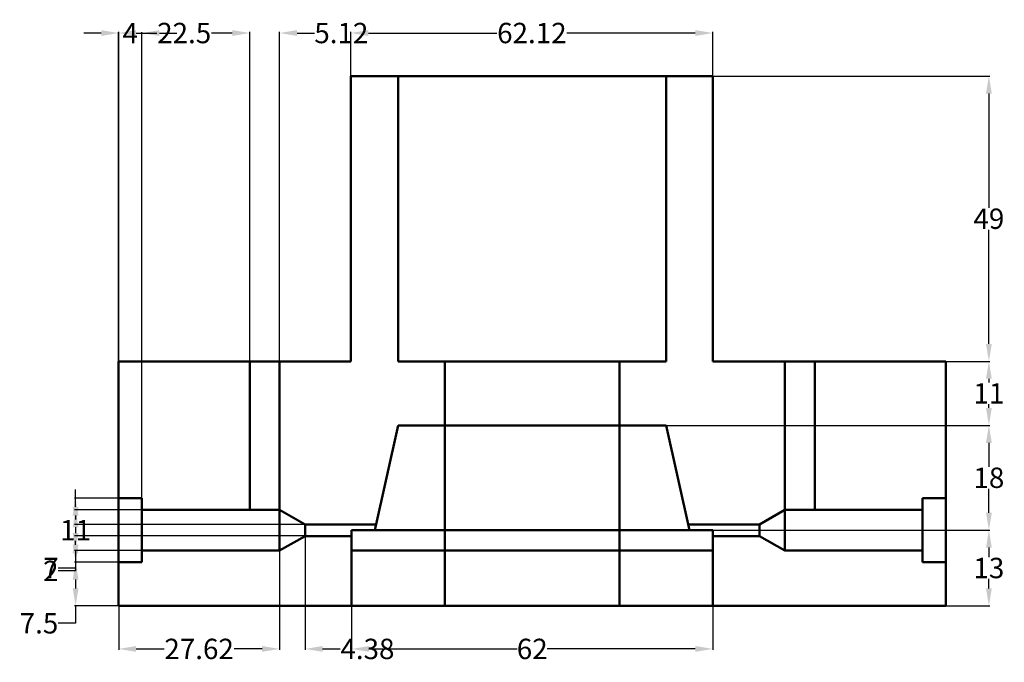
# Model space of a CAD drawing. Units: millimetres. Extents: x 646 to 860, y 238 to 552.
# Tile 1 of 2: x 646 to 815, y 238 to 349. Entities that reach past the tile are written whole.
import ezdxf

# ---------------------------------------------------------------- set-up
doc = ezdxf.new("R2010")
doc.units = ezdxf.units.MM
doc.header["$MEASUREMENT"] = 0
doc.layers.add('M-DIMS', color=2, linetype='Continuous', lineweight=18)
doc.layers.add('M-OUTL', color=7, linetype='Continuous', lineweight=50)
doc.styles.get("Standard").update_dxf_attribs({"font": 'arial.ttf'})
doc.dimstyles.get("Standard").update_dxf_attribs({"dimtxt": 3.5, "dimasz": 3, "dimexe": 0.18, "dimexo": 0.0625, "dimgap": 0.09, "dimtad": 0, "dimtih": 1, "dimtoh": 1, "dimdec": 1, "dimzin": 0, "dimdsep": 46, "dimtxsty": 'Standard', "dimcen": 0.09, "dimadec": 0, "dimazin": 0, "dimtfac": 1, "dimtdec": 1, "dimtofl": 0, "dimtmove": 0, "dimatfit": 3, "dimfxl": 1, "dimtolj": 1, "dimtzin": 0, "dimarcsym": 0})

# ---------------------------------------------------------------- blocks, each defined once
blk = doc.blocks.new('*D25')
at = {"layer": 'Defpoints', "color": 0, "transparency": 16777216}
for p in [(765.02, 261.19), (812.42, 261.19), (805.02, 248.19)]:
    blk.add_point(p, dxfattribs=at)
at = {"layer": 'M-DIMS', "color": 0, "lineweight": -2, "transparency": 16777216}
for p, q in [((765.08, 261.19), (812.6, 261.19)), ((812.42, 258.19), (812.42, 256.56)), ((812.42, 251.19), (812.42, 252.81)), ((805.08, 248.19), (812.6, 248.19))]:
    blk.add_line(p, q, dxfattribs=at)
at = {"layer": 'M-DIMS', "color": 0, "transparency": 16777216}
for points in [[(811.92, 258.19), (812.92, 258.19), (812.42, 261.19)], [(811.92, 251.19), (812.92, 251.19), (812.42, 248.19)]]:
    blk.add_solid(points, dxfattribs=at)
at = {"layer": 'M-DIMS', "color": 0, "transparency": 16777216, "insert": (812.42, 254.69), "char_height": 3.5, "attachment_point": 5}
blk.add_mtext('\\A1;13', dxfattribs=at)
blk = doc.blocks.new('*D26')
at = {"layer": 'Defpoints', "color": 0, "transparency": 16777216}
for p in [(757.02, 279.19), (812.42, 279.19), (765.02, 261.19)]:
    blk.add_point(p, dxfattribs=at)
at = {"layer": 'M-DIMS', "color": 0, "lineweight": -2, "transparency": 16777216}
for p, q in [((757.08, 279.19), (812.6, 279.19)), ((812.42, 276.19), (812.42, 272.06)), ((812.42, 264.19), (812.42, 268.31)), ((765.08, 261.19), (812.6, 261.19))]:
    blk.add_line(p, q, dxfattribs=at)
at = {"layer": 'M-DIMS', "color": 0, "transparency": 16777216}
for points in [[(811.92, 276.19), (812.92, 276.19), (812.42, 279.19)], [(811.92, 264.19), (812.92, 264.19), (812.42, 261.19)]]:
    blk.add_solid(points, dxfattribs=at)
at = {"layer": 'M-DIMS', "color": 0, "transparency": 16777216, "insert": (812.42, 270.19), "char_height": 3.5, "attachment_point": 5}
blk.add_mtext('\\A1;18', dxfattribs=at)
blk = doc.blocks.new('*D27')
at = {"layer": 'Defpoints', "color": 0, "transparency": 16777216}
for p in [(805.02, 290.19), (812.42, 290.19), (757.02, 279.19)]:
    blk.add_point(p, dxfattribs=at)
at = {"layer": 'M-DIMS', "color": 0, "lineweight": -2, "transparency": 16777216}
for p, q in [((805.08, 290.19), (812.6, 290.19)), ((812.42, 287.19), (812.42, 286.53)), ((812.42, 282.19), (812.42, 282.84)), ((757.08, 279.19), (812.6, 279.19))]:
    blk.add_line(p, q, dxfattribs=at)
at = {"layer": 'M-DIMS', "color": 0, "transparency": 16777216}
for points in [[(811.92, 287.19), (812.92, 287.19), (812.42, 290.19)], [(811.92, 282.19), (812.92, 282.19), (812.42, 279.19)]]:
    blk.add_solid(points, dxfattribs=at)
at = {"layer": 'M-DIMS', "color": 0, "transparency": 16777216, "insert": (812.42, 284.69), "char_height": 3.5, "attachment_point": 5}
blk.add_mtext('\\A1;11', dxfattribs=at)
blk = doc.blocks.new('*D28')
at = {"layer": 'Defpoints', "color": 0, "transparency": 16777216}
for p in [(765.02, 339.19), (812.42, 339.19), (805.02, 290.19)]:
    blk.add_point(p, dxfattribs=at)
at = {"layer": 'M-DIMS', "color": 0, "lineweight": -2, "transparency": 16777216}
for p, q in [((765.08, 339.19), (812.6, 339.19)), ((812.42, 336.19), (812.42, 316.56)), ((812.42, 293.19), (812.42, 312.81)), ((805.08, 290.19), (812.6, 290.19))]:
    blk.add_line(p, q, dxfattribs=at)
at = {"layer": 'M-DIMS', "color": 0, "transparency": 16777216}
for points in [[(811.92, 336.19), (812.92, 336.19), (812.42, 339.19)], [(811.92, 293.19), (812.92, 293.19), (812.42, 290.19)]]:
    blk.add_solid(points, dxfattribs=at)
at = {"layer": 'M-DIMS', "color": 0, "transparency": 16777216, "insert": (812.42, 314.69), "char_height": 3.5, "attachment_point": 5}
blk.add_mtext('\\A1;49', dxfattribs=at)
blk = doc.blocks.new('*D29')
at = {"layer": 'Defpoints', "color": 0, "transparency": 16777216}
for p in [(765.02, 346.59), (702.9, 339.19), (765.02, 339.19)]:
    blk.add_point(p, dxfattribs=at)
at = {"layer": 'M-DIMS', "color": 0, "lineweight": -2, "transparency": 16777216}
for p, q in [((702.9, 339.25), (702.9, 346.77)), ((705.9, 346.59), (727.97, 346.59)), ((762.02, 346.59), (739.94, 346.59)), ((765.02, 339.25), (765.02, 346.77))]:
    blk.add_line(p, q, dxfattribs=at)
at = {"layer": 'M-DIMS', "color": 0, "transparency": 16777216}
for points in [[(705.9, 347.09), (705.9, 346.09), (702.9, 346.59)], [(762.02, 347.09), (762.02, 346.09), (765.02, 346.59)]]:
    blk.add_solid(points, dxfattribs=at)
at = {"layer": 'M-DIMS', "color": 0, "transparency": 16777216, "insert": (733.96, 346.59), "char_height": 3.5, "attachment_point": 5}
blk.add_mtext('\\A1;62.12', dxfattribs=at)
blk = doc.blocks.new('*D30')
at = {"layer": 'Defpoints', "color": 0, "transparency": 16777216}
for p in [(703.02, 248.19), (765.02, 248.19), (765.02, 240.79)]:
    blk.add_point(p, dxfattribs=at)
at = {"layer": 'M-DIMS', "color": 0, "lineweight": -2, "transparency": 16777216}
for p, q in [((703.02, 248.12), (703.02, 240.61)), ((765.02, 248.12), (765.02, 240.61)), ((706.02, 240.79), (731.43, 240.79)), ((762.02, 240.79), (736.6, 240.79))]:
    blk.add_line(p, q, dxfattribs=at)
at = {"layer": 'M-DIMS', "color": 0, "transparency": 16777216}
for points in [[(706.02, 241.29), (706.02, 240.29), (703.02, 240.79)], [(762.02, 241.29), (762.02, 240.29), (765.02, 240.79)]]:
    blk.add_solid(points, dxfattribs=at)
at = {"layer": 'M-DIMS', "color": 0, "transparency": 16777216, "insert": (734.02, 240.79), "char_height": 3.5, "attachment_point": 5}
blk.add_mtext('\\A1;62', dxfattribs=at)
blk = doc.blocks.new('*D31')
at = {"layer": 'Defpoints', "color": 0, "transparency": 16777216}
for p in [(663.02, 266.69), (655.62, 255.69), (663.02, 255.69)]:
    blk.add_point(p, dxfattribs=at)
at = {"layer": 'M-DIMS', "color": 0, "lineweight": -2, "transparency": 16777216}
for p, q in [((662.95, 266.69), (655.44, 266.69)), ((655.62, 263.69), (655.62, 263.03)), ((655.62, 258.69), (655.62, 259.34)), ((662.95, 255.69), (655.44, 255.69))]:
    blk.add_line(p, q, dxfattribs=at)
at = {"layer": 'M-DIMS', "color": 0, "transparency": 16777216}
for points in [[(655.12, 263.69), (656.12, 263.69), (655.62, 266.69)], [(655.12, 258.69), (656.12, 258.69), (655.62, 255.69)]]:
    blk.add_solid(points, dxfattribs=at)
at = {"layer": 'M-DIMS', "color": 0, "transparency": 16777216, "insert": (655.62, 261.19), "char_height": 3.5, "attachment_point": 5}
blk.add_mtext('\\A1;11', dxfattribs=at)
blk = doc.blocks.new('*D32')
at = {"layer": 'Defpoints', "color": 0, "transparency": 16777216}
for p in [(667.015746, 346.585612), (663.015746, 266.685612), (667.015746, 266.685612)]:
    blk.add_point(p, dxfattribs=at)
at = {"layer": 'M-DIMS', "color": 0, "lineweight": -2, "transparency": 16777216}
for p, q in [((660.015746, 346.585612), (657.015746, 346.585612)), ((663.015746, 266.748112), (663.015746, 346.765612)), ((667.015746, 266.748112), (667.015746, 346.765612)), ((670.015746, 346.585612), (673.015746, 346.585612))]:
    blk.add_line(p, q, dxfattribs=at)
at = {"layer": 'M-DIMS', "color": 0, "transparency": 16777216}
for points in [[(660.015746, 347.085612), (660.015746, 346.085612), (663.015746, 346.585612)], [(670.015746, 347.085612), (670.015746, 346.085612), (667.015746, 346.585612)]]:
    blk.add_solid(points, dxfattribs=at)
at = {"layer": 'M-DIMS', "color": 0, "transparency": 16777216, "insert": (665.015746, 346.585612), "char_height": 3.5, "attachment_point": 5}
blk.add_mtext('\\A1;4', dxfattribs=at)
blk = doc.blocks.new('*D33')
at = {"layer": 'Defpoints', "color": 0, "transparency": 16777216}
for p in [(667.02, 264.69), (655.62, 257.69), (667.02, 257.69)]:
    blk.add_point(p, dxfattribs=at)
at = {"layer": 'M-DIMS', "color": 0, "lineweight": -2, "transparency": 16777216}
for p, q in [((666.95, 264.69), (655.44, 264.69)), ((655.62, 261.69), (655.62, 260.69)), ((666.95, 257.69), (655.44, 257.69)), ((655.62, 257.69), (655.62, 254.69)), ((655.62, 254.69), (652.62, 254.69))]:
    blk.add_line(p, q, dxfattribs=at)
at = {"layer": 'M-DIMS', "color": 0, "transparency": 16777216}
for points in [[(655.12, 261.69), (656.12, 261.69), (655.62, 264.69)], [(655.12, 260.69), (656.12, 260.69), (655.62, 257.69)]]:
    blk.add_solid(points, dxfattribs=at)
at = {"layer": 'M-DIMS', "color": 0, "transparency": 16777216, "insert": (651.39, 254.69), "char_height": 3.5, "attachment_point": 5}
blk.add_mtext('\\A1;7', dxfattribs=at)
blk = doc.blocks.new('*D34')
at = {"layer": 'Defpoints', "color": 0, "transparency": 16777216}
for p in [(690.64, 257.69), (663.02, 255.69), (690.64, 240.79)]:
    blk.add_point(p, dxfattribs=at)
at = {"layer": 'M-DIMS', "color": 0, "lineweight": -2, "transparency": 16777216}
for p, q in [((690.64, 257.62), (690.64, 240.61)), ((663.02, 255.62), (663.02, 240.61)), ((666.02, 240.79), (670.82, 240.79)), ((687.64, 240.79), (682.83, 240.79))]:
    blk.add_line(p, q, dxfattribs=at)
at = {"layer": 'M-DIMS', "color": 0, "transparency": 16777216}
for points in [[(666.02, 241.29), (666.02, 240.29), (663.02, 240.79)], [(687.64, 241.29), (687.64, 240.29), (690.64, 240.79)]]:
    blk.add_solid(points, dxfattribs=at)
at = {"layer": 'M-DIMS', "color": 0, "transparency": 16777216, "insert": (676.83, 240.79), "char_height": 3.5, "attachment_point": 5}
blk.add_mtext('\\A1;27.62', dxfattribs=at)
blk = doc.blocks.new('*D35')
at = {"layer": 'Defpoints', "color": 0, "transparency": 16777216}
for p in [(690.64, 264.69), (695.02, 262.19), (695.02, 240.79)]:
    blk.add_point(p, dxfattribs=at)
at = {"layer": 'M-DIMS', "color": 0, "lineweight": -2, "transparency": 16777216}
for p, q in [((690.64, 264.62), (690.64, 240.61)), ((695.02, 262.12), (695.02, 240.61)), ((687.64, 240.79), (684.64, 240.79)), ((698.02, 240.79), (701.02, 240.79))]:
    blk.add_line(p, q, dxfattribs=at)
at = {"layer": 'M-DIMS', "color": 0, "transparency": 16777216}
for points in [[(687.64, 241.29), (687.64, 240.29), (690.64, 240.79)], [(698.02, 241.29), (698.02, 240.29), (695.02, 240.79)]]:
    blk.add_solid(points, dxfattribs=at)
at = {"layer": 'M-DIMS', "color": 0, "transparency": 16777216, "insert": (705.73, 240.79), "char_height": 3.5, "attachment_point": 5}
blk.add_mtext('\\A1;4.38', dxfattribs=at)
blk = doc.blocks.new('*D36')
at = {"layer": 'Defpoints', "color": 0, "transparency": 16777216}
for p in [(695.02, 262.19), (655.62, 260.19), (695.02, 260.19)]:
    blk.add_point(p, dxfattribs=at)
at = {"layer": 'M-DIMS', "color": 0, "lineweight": -2, "transparency": 16777216}
for p, q in [((655.62, 265.19), (655.62, 268.19)), ((694.95, 262.19), (655.44, 262.19)), ((694.95, 260.19), (655.44, 260.19)), ((655.62, 257.19), (655.62, 254.19)), ((655.62, 254.19), (652.62, 254.19))]:
    blk.add_line(p, q, dxfattribs=at)
at = {"layer": 'M-DIMS', "color": 0, "transparency": 16777216}
for points in [[(655.12, 265.19), (656.12, 265.19), (655.62, 262.19)], [(655.12, 257.19), (656.12, 257.19), (655.62, 260.19)]]:
    blk.add_solid(points, dxfattribs=at)
at = {"layer": 'M-DIMS', "color": 0, "transparency": 16777216, "insert": (651.37, 254.19), "char_height": 3.5, "attachment_point": 5}
blk.add_mtext('\\A1;2', dxfattribs=at)
blk = doc.blocks.new('*D37')
at = {"layer": 'Defpoints', "color": 0, "transparency": 16777216}
for p in [(663.02, 255.69), (655.62, 248.19), (663.02, 248.19)]:
    blk.add_point(p, dxfattribs=at)
at = {"layer": 'M-DIMS', "color": 0, "lineweight": -2, "transparency": 16777216}
for p, q in [((662.95, 255.69), (655.44, 255.69)), ((655.62, 252.69), (655.62, 251.19)), ((662.95, 248.19), (655.44, 248.19)), ((655.62, 248.19), (655.62, 245.19)), ((655.62, 245.19), (652.62, 245.19))]:
    blk.add_line(p, q, dxfattribs=at)
at = {"layer": 'M-DIMS', "color": 0, "transparency": 16777216}
for points in [[(655.12, 252.69), (656.12, 252.69), (655.62, 255.69)], [(655.12, 251.19), (656.12, 251.19), (655.62, 248.19)]]:
    blk.add_solid(points, dxfattribs=at)
at = {"layer": 'M-DIMS', "color": 0, "transparency": 16777216, "insert": (649.34, 245.19), "char_height": 3.5, "attachment_point": 5}
blk.add_mtext('\\A1;7.5', dxfattribs=at)
blk = doc.blocks.new('*D38')
at = {"layer": 'Defpoints', "color": 0, "transparency": 16777216}
for p in [(690.64, 346.59), (685.52, 290.19), (690.64, 290.19)]:
    blk.add_point(p, dxfattribs=at)
at = {"layer": 'M-DIMS', "color": 0, "lineweight": -2, "transparency": 16777216}
for p, q in [((682.52, 346.59), (679.52, 346.59)), ((685.52, 290.25), (685.52, 346.77)), ((690.64, 290.25), (690.64, 346.77)), ((693.64, 346.59), (696.64, 346.59))]:
    blk.add_line(p, q, dxfattribs=at)
at = {"layer": 'M-DIMS', "color": 0, "transparency": 16777216}
for points in [[(682.52, 347.09), (682.52, 346.09), (685.52, 346.59)], [(693.64, 347.09), (693.64, 346.09), (690.64, 346.59)]]:
    blk.add_solid(points, dxfattribs=at)
at = {"layer": 'M-DIMS', "color": 0, "transparency": 16777216, "insert": (701.25, 346.59), "char_height": 3.5, "attachment_point": 5}
blk.add_mtext('\\A1;5.12', dxfattribs=at)
blk = doc.blocks.new('*D39')
at = {"layer": 'Defpoints', "color": 0, "transparency": 16777216}
for p in [(685.52, 346.59), (663.02, 290.19), (685.52, 290.19)]:
    blk.add_point(p, dxfattribs=at)
at = {"layer": 'M-DIMS', "color": 0, "lineweight": -2, "transparency": 16777216}
for p, q in [((663.02, 290.25), (663.02, 346.77)), ((666.02, 346.59), (669.59, 346.59)), ((682.52, 346.59), (678.94, 346.59)), ((685.52, 290.25), (685.52, 346.77))]:
    blk.add_line(p, q, dxfattribs=at)
at = {"layer": 'M-DIMS', "color": 0, "transparency": 16777216}
for points in [[(666.02, 347.09), (666.02, 346.09), (663.02, 346.59)], [(682.52, 347.09), (682.52, 346.09), (685.52, 346.59)]]:
    blk.add_solid(points, dxfattribs=at)
at = {"layer": 'M-DIMS', "color": 0, "transparency": 16777216, "insert": (674.27, 346.59), "char_height": 3.5, "attachment_point": 5}
blk.add_mtext('\\A1;22.5', dxfattribs=at)

msp = doc.modelspace()

# ---------------------------------------------------------------- linework, layer by layer
at = {"layer": 'M-OUTL'}
for p, q in [((765.016, 339.186), (702.896, 339.186)), ((702.896, 290.186), (702.896, 339.186)), ((711.016, 290.186), (711.016, 339.186)), ((757.016, 290.186), (757.016, 339.186)), ((765.016, 290.186), (765.016, 339.186)), ((663.016, 290.186), (663.016, 248.186)), ((690.636, 290.186), (663.016, 290.186)), ((685.516, 290.186), (685.516, 264.686)), ((702.896, 290.186), (690.636, 290.186)), ((690.636, 290.186), (690.636, 257.686)), ((757.016, 290.186), (711.016, 290.186)), ((719.016, 290.186), (719.016, 248.186)), ((749.016, 290.186), (749.016, 248.186)), ((805.016, 290.186), (765.016, 290.186)), ((777.396, 290.186), (777.396, 257.686)), ((782.516, 290.186), (782.516, 264.686)), ((805.016, 290.186), (805.016, 248.186)), ((711.016, 279.186), (707.016, 261.186)), ((757.016, 279.186), (711.016, 279.186)), ((749.016, 279.186), (757.016, 279.186)), ((757.016, 279.186), (761.016, 261.186)), ((663.016, 266.686), (667.016, 266.686)), ((667.016, 266.686), (667.016, 255.686)), ((801.016, 266.686), (801.016, 255.686)), ((805.016, 266.686), (801.016, 266.686)), ((667.016, 264.686), (690.636, 264.686)), ((690.636, 264.686), (690.636, 257.686)), ((695.016, 262.186), (690.636, 264.686)), ((773.016, 262.186), (777.396, 264.686)), ((801.016, 264.686), (777.396, 264.686)), ((695.016, 262.186), (707.238, 262.186)), ((695.016, 260.186), (695.016, 262.186)), ((773.016, 262.186), (760.794, 262.186)), ((773.016, 260.186), (773.016, 262.186)), ((703.016, 261.186), (703.016, 248.186)), ((703.016, 261.186), (757.016, 261.186)), ((765.016, 261.186), (711.016, 261.186)), ((765.016, 261.186), (765.016, 248.186)), ((695.016, 260.186), (690.636, 257.686)), ((695.016, 260.186), (703.016, 260.186)), ((773.016, 260.186), (765.016, 260.186)), ((773.016, 260.186), (777.396, 257.686)), ((667.016, 257.686), (690.636, 257.686)), ((667.016, 257.686), (690.636, 257.686)), ((703.016, 257.686), (757.016, 257.686)), ((765.016, 257.686), (711.016, 257.686)), ((801.016, 257.686), (777.396, 257.686)), ((801.016, 257.686), (777.396, 257.686)), ((663.016, 255.686), (667.016, 255.686)), ((805.016, 255.686), (801.016, 255.686)), ((663.016, 248.186), (749.016, 248.186)), ((805.016, 248.186), (749.016, 248.186))]:
    msp.add_line(p, q, dxfattribs=at)

# ---------------------------------------------------------------- dimensions: what is measured, and where the dimension line sits
at = {"layer": 'M-DIMS'}
for base, p1, p2, override, picture, middle in [((667.016, 346.586), (663.016, 266.686), (667.016, 266.686), {"dimdec": 0, "dimlfac": 1, "dimrnd": 0, "dimzin": 0, "dimdsep": 46, "dimlunit": 2}, '*D32', (665.016, 346.586)), ((685.516, 346.586), (663.016, 290.186), (685.516, 290.186), {"dimdec": 1, "dimlfac": 1, "dimrnd": 0, "dimzin": 0, "dimdsep": 46, "dimlunit": 2}, '*D39', (674.266, 346.586)), ((690.636, 346.586), (685.516, 290.186), (690.636, 290.186), {"dimdec": 2, "dimlfac": 1, "dimrnd": 0, "dimzin": 0, "dimdsep": 46, "dimlunit": 2}, '*D38', (701.254, 346.586)), ((765.016, 346.586), (702.896, 339.186), (765.016, 339.186), {"dimdec": 2, "dimlfac": 1, "dimrnd": 0, "dimzin": 0, "dimdsep": 46, "dimlunit": 2}, '*D29', (733.956, 346.586)), ((695.016, 240.786), (690.636, 264.686), (695.016, 262.186), {"dimdec": 2, "dimlfac": 1, "dimrnd": 0, "dimzin": 0, "dimdsep": 46, "dimlunit": 2}, '*D35', (705.725, 240.786)), ((690.636, 240.786), (663.016, 255.686), (690.636, 257.686), {"dimdec": 2, "dimlfac": 1, "dimrnd": 0, "dimzin": 0, "dimdsep": 46, "dimlunit": 2}, '*D34', (676.826, 240.786)), ((765.016, 240.786), (703.016, 248.186), (765.016, 248.186), {"dimdec": 0, "dimlfac": 1, "dimrnd": 0, "dimzin": 0, "dimdsep": 46, "dimlunit": 2}, '*D30', (734.016, 240.786))]:
    dim = msp.add_linear_dim(base=base, p1=p1, p2=p2, dimstyle='Standard', override=override, dxfattribs=at)
    dim.commit()
    dim.dimension.update_dxf_attribs({"geometry": picture, "text_midpoint": middle})
for base, p1, p2, override, picture, middle in [((812.416, 339.186), (805.016, 290.186), (765.016, 339.186), {"dimdec": 0, "dimlfac": 1, "dimrnd": 0, "dimzin": 0, "dimdsep": 46, "dimlunit": 2}, '*D28', (812.416, 314.686)), ((812.416, 290.186), (757.016, 279.186), (805.016, 290.186), {"dimdec": 0, "dimlfac": 1, "dimrnd": 0, "dimzin": 0, "dimdsep": 46, "dimlunit": 2}, '*D27', (812.416, 284.686)), ((812.416, 279.186), (765.016, 261.186), (757.016, 279.186), {"dimdec": 0, "dimlfac": 1, "dimrnd": 0, "dimzin": 0, "dimdsep": 46, "dimlunit": 2}, '*D26', (812.416, 270.186)), ((655.616, 260.186), (695.016, 262.186), (695.016, 260.186), {"dimdec": 0, "dimlfac": 1, "dimrnd": 0, "dimzin": 0, "dimdsep": 46, "dimlunit": 2}, '*D36', (651.367, 254.186)), ((655.616, 255.686), (663.016, 266.686), (663.016, 255.686), {"dimdec": 0, "dimlfac": 1, "dimrnd": 0, "dimzin": 0, "dimdsep": 46, "dimlunit": 2}, '*D31', (655.616, 261.186)), ((655.616, 257.686), (667.016, 264.686), (667.016, 257.686), {"dimdec": 0, "dimlfac": 1, "dimrnd": 0, "dimzin": 0, "dimdsep": 46, "dimlunit": 2}, '*D33', (651.393, 254.686)), ((812.416, 261.186), (805.016, 248.186), (765.016, 261.186), {"dimdec": 0, "dimlfac": 1, "dimrnd": 0, "dimzin": 0, "dimdsep": 46, "dimlunit": 2}, '*D25', (812.416, 254.686)), ((655.616, 248.186), (663.016, 255.686), (663.016, 248.186), {"dimdec": 1, "dimlfac": 1, "dimrnd": 0, "dimzin": 0, "dimdsep": 46, "dimlunit": 2}, '*D37', (649.341, 245.186))]:
    dim = msp.add_linear_dim(base=base, p1=p1, p2=p2, angle=90, dimstyle='Standard', override=override, dxfattribs=at)
    dim.commit()
    dim.dimension.update_dxf_attribs({"geometry": picture, "text_midpoint": middle})

doc.saveas('drawing.dxf')
